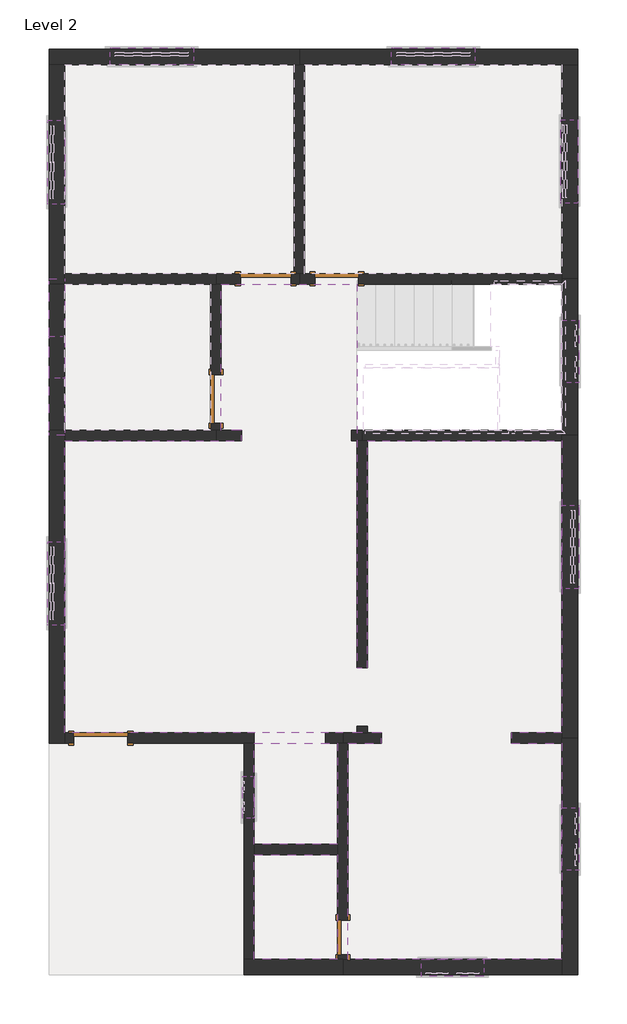
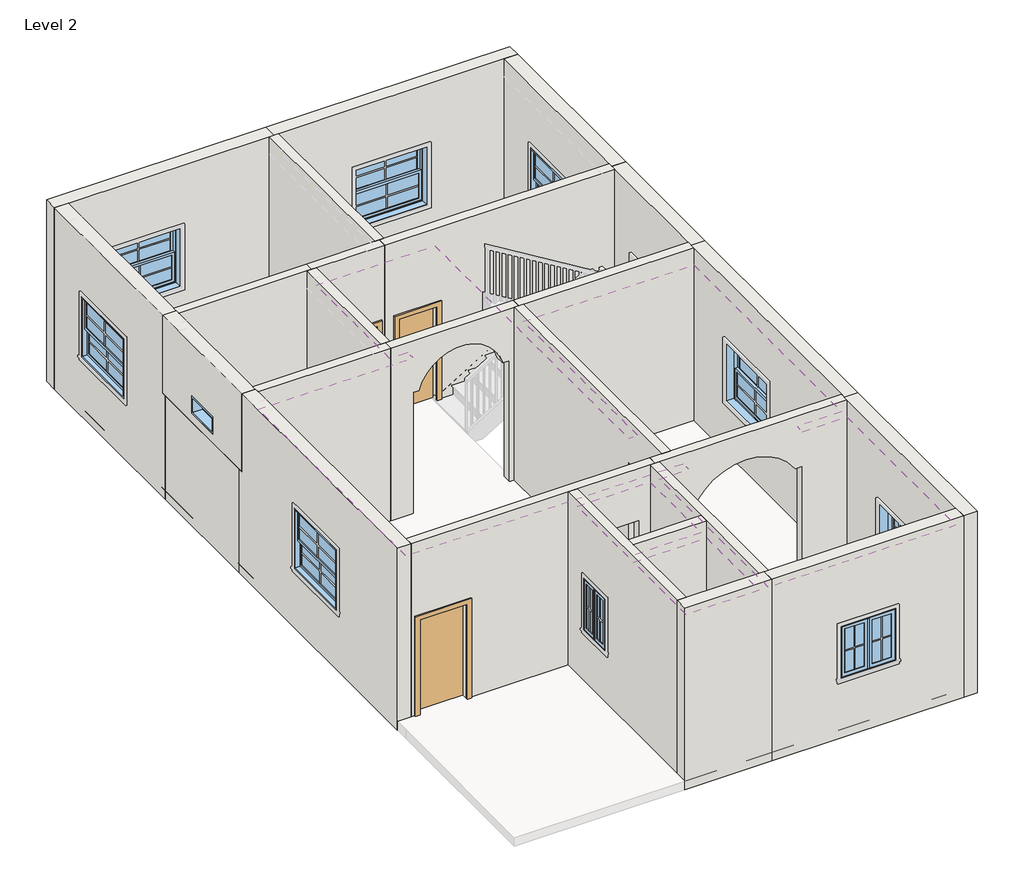
# One storey, part 1 of 2: 26 walls, 11 windows, 5 doors, 3 coverings.
# Revit data of these elements (continued)
# Element 15 (IfcWall, "Generic - 6\"")
#   built-in parameter 1001111 = 0' - 6"
#   Top Offset = 0' - 0"
#   Base Offset = 0' - 6"
#   Unconnected Height = 10' - 6"
#   wall height = 10' - 6"
#   Phase Created = New Construction
#   Base Constraint = Level 2
#   Materials on its faces: "Default Wall", "GOLD"
# Element 18 (IfcWall, "Generic - 6\"")
#   built-in parameter 1001111 = 0' - 6"
#   Top Offset = 0' - 0"
#   Base Offset = 0' - 6"
#   Unconnected Height = 10' - 6"
#   wall height = 10' - 6"
#   Phase Created = New Construction
#   Base Constraint = Level 2
#   Materials on its faces: "Default Wall", "DINING ROOM WALL", "LAVENDER WHITE"
# Elements 19, 21 (IfcWall, "Generic - 6\"")
#   built-in parameter 1001111 = 0' - 6"
#   Top Offset = 0' - 0"
#   Base Offset = 0' - 6"
#   Unconnected Height = 10' - 6"
#   wall height = 10' - 6"
#   Phase Created = New Construction
#   Base Constraint = Level 2
#   Materials on its faces: "Default Wall", "DINING ROOM WALL"
# Element 20 (IfcWall, "Generic - 6\"")
#   built-in parameter 1001111 = 0' - 6"
#   Top Offset = 0' - 0"
#   Base Offset = 0' - 6"
#   Unconnected Height = 10' - 6"
#   wall height = 10' - 6"
#   Phase Created = New Construction
#   Base Constraint = Level 2
#   Materials on its faces: "Default Wall", "LIVING ROOM WALL"
# Element 23 (IfcWall, "Generic - 9\"")
#   built-in parameter 1001111 = 0' - 6"
#   Top Offset = 0' - 0"
#   Base Offset = 0' - 6"
#   Unconnected Height = 10' - 6"
#   wall height = 10' - 6"
#   Phase Created = New Construction
#   Base Constraint = Level 2
#   Materials on its faces: "Default Wall", "BURGUNDY COLOUR"
# Elements 24, 26 (IfcWall, "Generic - 9\"")
#   built-in parameter 1001111 = 0' - 6"
#   Top Offset = 0' - 0"
#   Base Offset = 0' - 6"
#   Unconnected Height = 10' - 6"
#   wall height = 10' - 6"
#   Phase Created = New Construction
#   Base Constraint = Level 2
#   Materials on its faces: "Default Wall", "LAVENDER WHITE"
# Element 25 (IfcWall, "Generic - 9\"")
#   built-in parameter 1001111 = 0' - 6"
#   Top Offset = 0' - 0"
#   Base Offset = 0' - 6"
#   Unconnected Height = 10' - 6"
#   wall height = 10' - 6"
#   Phase Created = New Construction
#   Base Constraint = Level 2
#   Materials on its faces: "Default Wall", "GOLD"
# Elements 27, 28, 29, 31, 32 (IfcWall, "Generic - 9\"")
#   built-in parameter 1001111 = 0' - 6"
#   Top Offset = 0' - 0"
#   Base Offset = 0' - 6"
#   Unconnected Height = 10' - 6"
#   wall height = 10' - 6"
#   Phase Created = New Construction
#   Base Constraint = Level 2
#   Materials on its faces: "Default Wall"
# Element 30 (IfcWall, "Generic - 9\"")
#   built-in parameter 1001111 = 0' - 6"
#   Top Offset = 0' - 0"
#   Base Offset = 0' - 6"
#   Unconnected Height = 10' - 6"
#   wall height = 10' - 6"
#   Phase Created = New Construction
#   Base Constraint = Level 2
#   Materials on its faces: "Default Wall", "DINING ROOM WALL"
# Element 33 (IfcWall, "Generic - 9\"")
#   built-in parameter 1001111 = 6' - 6"
#   Top Offset = 0' - 0"
#   Base Offset = 6' - 6"
#   Unconnected Height = 4' - 6"
#   wall height = 4' - 6"
#   Phase Created = New Construction
#   Base Constraint = Level 2
#   Materials on its faces: "Default Wall", "BATHROOM TILES"
# Element 34 (IfcWall, "Generic - 9\"")
#   built-in parameter 1001111 = 0' - 6"
#   Top Offset = 0' - 0"
#   Base Offset = 0' - 6"
#   Unconnected Height = 6' - 0"
#   wall height = 6' - 0"
#   Phase Created = New Construction
#   Base Constraint = Level 2
#   Materials on its faces: "Default Wall", "BATHROOM TILES"
# Element 35 (IfcWindow, "Fixed : 2'")
#   Mark = "21"
#   Phase Created = New Construction
#   Materials on its faces: "Sash", "Glass"
# Element 36 (IfcWindow, "Window-Casement-Double : 2'")
#   Mark = "20"
#   Window Inset = 0' - 0"
#   Interior Wall Closure = 0' - 2 1/4"
#   Frame Extension = 0' - 0 1/4"
#   Exterior Wall Closure = 0' - 1 1/4"
#   Interior Trim Visibility = yes
#   Exterior Trim Visibility = yes
#   Phase Created = New Construction
#   Materials on its faces: "Wood - Stained", "Glass", "Clad - White"
# Element 37 (IfcWindow, "Window-Casement-Double : 3'")
#   Mark = "18"
#   Window Inset = 0' - 0"
#   Interior Wall Closure = 0' - 2 1/4"
#   Frame Extension = 0' - 0 1/4"
#   Exterior Wall Closure = 0' - 1 1/4"
#   Interior Trim Visibility = yes
#   Exterior Trim Visibility = yes
#   Phase Created = New Construction
#   Materials on its faces: "Wood - Stained", "Glass", "Clad - White"
# Element 38 (IfcWindow, "Window-Casement-Double : 3'")
#   Mark = "19"
#   Window Inset = 0' - 0"
#   Interior Wall Closure = 0' - 2 1/4"
#   Frame Extension = 0' - 0 1/4"
#   Exterior Wall Closure = 0' - 1 1/4"
#   Interior Trim Visibility = yes
#   Exterior Trim Visibility = yes
#   Phase Created = New Construction
#   Materials on its faces: "Wood - Stained", "Glass", "Clad - White"
# Element 39 (IfcWindow, "Window-Casement-Double : 3'")
#   Mark = "22"
#   Window Inset = 0' - 0"
#   Interior Wall Closure = 0' - 2 1/4"
#   Frame Extension = 0' - 0 1/4"
#   Exterior Wall Closure = 0' - 1 1/4"
#   Interior Trim Visibility = yes
#   Exterior Trim Visibility = yes
#   Phase Created = New Construction
#   Materials on its faces: "Wood - Stained", "Glass", "Clad - White"
# Element 40 (IfcWindow, "Window-Double-Hung : 4'")
#   Mark = "14"
#   Window Inset = 0' - 0"
#   Interior Wall Closure = 0' - 1 1/2"
#   Frame Extension = 0' - 1 1/4"
#   Exterior Wall Closure = 0' - 0 1/2"
#   Interior Trim Visibility = yes
#   Indicator Visibility = yes
#   Exterior Trim Visibility = yes
#   Phase Created = New Construction
#   Materials on its faces: "Wood - Stained", "Glass", "Clad - White"
# Element 41 (IfcWindow, "Window-Double-Hung : 4'")
#   Mark = "16"
#   Window Inset = 0' - 0"
#   Interior Wall Closure = 0' - 1 1/2"
#   Frame Extension = 0' - 1 1/4"
#   Exterior Wall Closure = 0' - 0 1/2"
#   Interior Trim Visibility = yes
#   Indicator Visibility = yes
#   Exterior Trim Visibility = yes
#   Phase Created = New Construction
#   Materials on its faces: "Wood - Stained", "Glass", "Clad - White"
# Element 42 (IfcWindow, "Window-Double-Hung : 4'")
#   Mark = "17"
#   Window Inset = 0' - 0"
#   Interior Wall Closure = 0' - 1 1/2"
#   Frame Extension = 0' - 1 1/4"
#   Exterior Wall Closure = 0' - 0 1/2"
#   Interior Trim Visibility = yes
#   Indicator Visibility = yes
#   Exterior Trim Visibility = yes
#   Phase Created = New Construction
#   Materials on its faces: "Wood - Stained", "Glass", "Clad - White"
# Element 43 (IfcWindow, "Window-Double-Hung : 4'")
#   Mark = "12"
#   Window Inset = 0' - 0"
#   Interior Wall Closure = 0' - 1 1/2"
#   Frame Extension = 0' - 1 1/4"
#   Exterior Wall Closure = 0' - 0 1/2"
#   Interior Trim Visibility = yes
#   Indicator Visibility = yes
#   Exterior Trim Visibility = yes
#   Phase Created = New Construction
#   Materials on its faces: "Wood - Stained", "Glass", "Clad - White"
# Element 44 (IfcWindow, "Window-Double-Hung : 4'")
#   Mark = "13"
#   Window Inset = 0' - 0"
#   Interior Wall Closure = 0' - 1 1/2"
#   Frame Extension = 0' - 1 1/4"
#   Exterior Wall Closure = 0' - 0 1/2"
#   Interior Trim Visibility = yes
#   Indicator Visibility = yes
#   Exterior Trim Visibility = yes
#   Phase Created = New Construction
#   Materials on its faces: "Wood - Stained", "Glass", "Clad - White"
# Element 45 (IfcWindow, "Window-Double-Hung : 4'")
#   Mark = "15"
#   Window Inset = 0' - 0"
#   Interior Wall Closure = 0' - 1 1/2"
#   Frame Extension = 0' - 1 1/4"
#   Exterior Wall Closure = 0' - 0 1/2"
#   Interior Trim Visibility = yes
#   Indicator Visibility = yes
#   Exterior Trim Visibility = yes
#   Phase Created = New Construction
#   Materials on its faces: "Wood - Stained", "Glass", "Clad - White"
# Materials
#   "Default": colour RGB 127 127 127, transparency 0, Cost = 0
#   "Acoustic Ceiling Tile 24 x 48": class "Generic", colour RGB 229 229 229, transparency 0, Description = "Acoustic Ceiling Tile 24 x 48", Cost = 0
#   "Door - Panel": class "Wood", colour RGB 210 159 95, transparency 0, Cost = 0
#   "Door - Frame": colour RGB 118 70 51, transparency 0, Cost = 0
#   "Glass": class "Glass", colour RGB 0 128 192, transparency 0.75, Description = "Soda Lime Glass", Cost = 0
#   "Sash": class "Wood", colour RGB 224 178 126, transparency 0, Cost = 0
#   "Wood - Stained": class "Wood", colour RGB 224 178 126, transparency 0, Cost = 0
#   "Clad - White": class "Wood", colour RGB 242 242 238, transparency 0, Cost = 0
#   "Default Wall": colour RGB 128 128 128, transparency 0, Cost = 0
#   "LAVENDER WHITE": class "Generic", colour RGB 120 120 120, transparency 0, Cost = 0
#   "LIVING ROOM WALL": class "Generic", colour RGB 120 120 120, transparency 0, Cost = 0
#   "BURGUNDY COLOUR": class "Generic", colour RGB 120 120 120, transparency 0, Cost = 0
#   "DINING ROOM WALL": class "Generic", colour RGB 120 120 120, transparency 0, Cost = 0
#   "GOLD": class "Generic", colour RGB 120 120 120, transparency 0, Cost = 0
#   "BATHROOM TILES": class "Generic", colour RGB 120 120 120, transparency 0, Cost = 0
